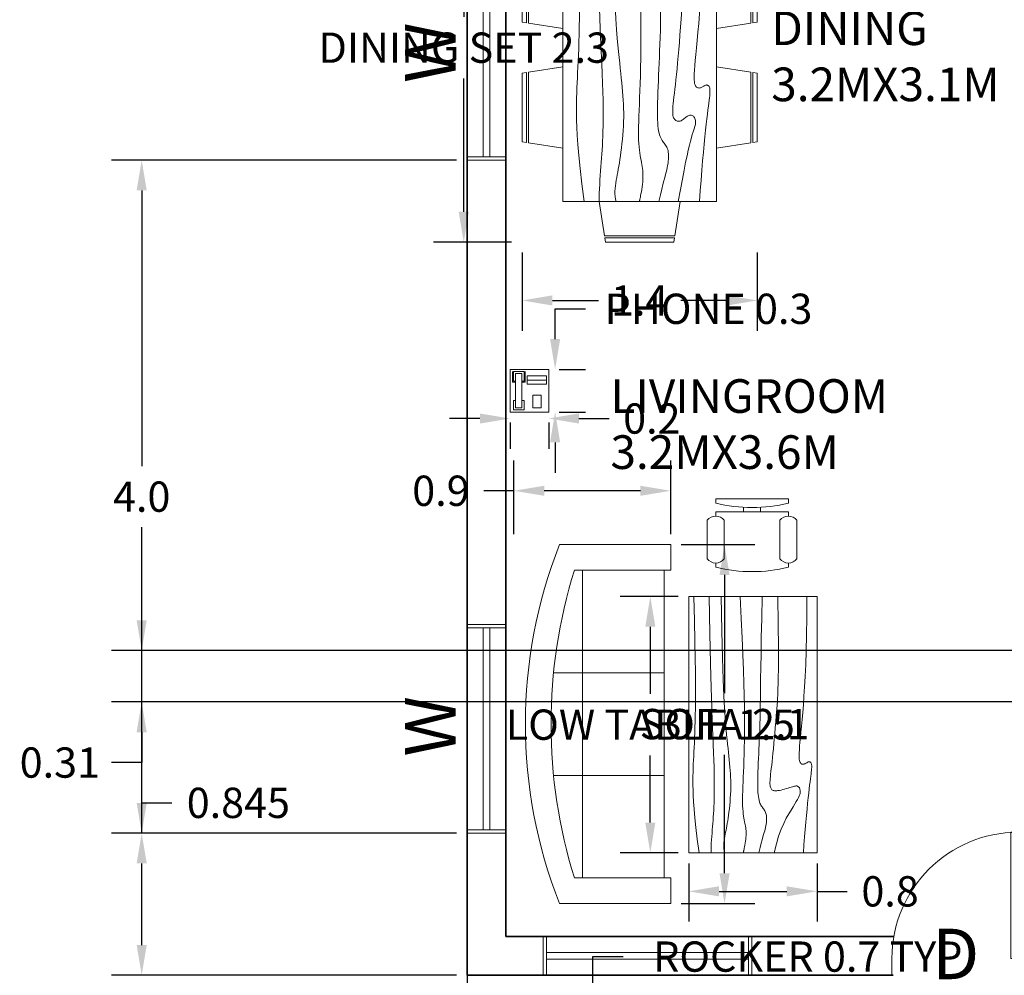
# Model space of a CAD drawing. Units: metres. Extents: x 40.9 to 56.1, y -1.4 to 24.2.
# Tile 3 of 7: x 42.6 to 48.4, y 12.9 to 18.6. Entities that reach past the tile are written whole.
import ezdxf

# ---------------------------------------------------------------- set-up
doc = ezdxf.new("R2010")
doc.units = ezdxf.units.M
doc.header["$MEASUREMENT"] = 0
for name, color, linetype, lineweight in [('A-ANNO-DIMS', 2, 'Continuous', 18), ('A-ANNO-TEXT', 7, 'Continuous', 18), ('A-AREA-IDEN', 7, 'Continuous', 18), ('A-DOOR', 3, 'Continuous', 18), ('A-EQPM', 8, 'Continuous', 18), ('A-FLOR', 7, 'Continuous', 25), ('A-FURN', 8, 'Continuous', 18), ('A-GLAZ', 4, 'Continuous', 18), ('A-WALL', 7, 'Continuous', 35)]:
    doc.layers.add(name, color=color, linetype=linetype, lineweight=lineweight)
doc.styles.get("Standard").update_dxf_attribs({"font": 'arial.ttf'})
doc.dimstyles.get("Standard").update_dxf_attribs({"dimtxt": 0.18, "dimasz": 0.18, "dimexe": 0.18, "dimexo": 0.0625, "dimgap": 0.09, "dimtad": 0, "dimtih": 1, "dimtoh": 1, "dimdec": 1, "dimzin": 0, "dimdsep": 46, "dimtxsty": 'Standard', "dimcen": 0.09, "dimadec": 0, "dimazin": 0, "dimtfac": 1, "dimtdec": 1, "dimtofl": 0, "dimtmove": 0, "dimatfit": 3, "dimfxl": 1, "dimtolj": 1, "dimtzin": 0, "dimarcsym": 0})

# ---------------------------------------------------------------- blocks, each defined once
blk = doc.blocks.new('*U3')
for p, q in [((-750, 0), (-750, -100)), ((0, 0), (0, -100))]:
    blk.add_line(p, q)
blk.add_lwpolyline([(0, 0), (0, 750), (-43.75, 750), (-43.75, 0)], close=True)
blk.add_arc((0, 0), 750, 90, 180)
blk = doc.blocks.new('Dining Set - 36 x 72 in.')
for p, q in [((-22.2343, 26.00059), (-23.4847, 17.99762)), ((-22.2304, 26), (-5.7608, 26)), ((-22, 27.5), (-22.1562, 26.50042)), ((-5.8416, 26.5), (-22.1534, 26.5)), ((-22, 27.5), (-6, 27.5)), ((-5.8437, 26.49966), (-6, 27.5)), ((-4.5152, 17.99762), (-5.7655, 25.99926)), ((5.7657, 26.00059), (4.5153, 17.99762)), ((5.7696, 26), (22.2392, 26)), ((6, 27.5), (5.8438, 26.50042)), ((22.1584, 26.5), (5.8466, 26.5)), ((6, 27.5), (22, 27.5)), ((22.1563, 26.49966), (22, 27.5)), ((23.4848, 17.99762), (22.2345, 25.99926)), ((36, 18), (-36, 18)), ((-36, 18), (-36, -18)), ((36, -18), (36, 18)), ((-44.0006, 8.23428), (-35.9976, 9.48474)), ((44.0006, 8.23428), (35.9976, 9.48474)), ((-45.5, 8), (-44.5004, 8.15617)), ((-45.5, 8), (-45.5, -8)), ((-44.5, -8.15843), (-44.5, 8.15338)), ((-44, 8.23041), (-44, -8.23915)), ((44, 8.23041), (44, -8.23915)), ((44.5, -8.15843), (44.5, 8.15338)), ((45.5, 8), (44.5005, 8.15617)), ((45.5, 8), (45.5, -8)), ((-44.4997, -8.15631), (-45.5, -8)), ((-35.9976, -9.48476), (-43.9993, -8.2345)), ((35.9976, -9.48476), (43.9993, -8.2345)), ((44.4997, -8.15631), (45.5, -8)), ((-36, -18), (36, -18)), ((-22.2343, -26.0006), (-23.4847, -17.99762)), ((-4.5152, -17.99762), (-5.7655, -25.99928)), ((5.7657, -26.0006), (4.5153, -17.99762)), ((23.4848, -17.99762), (22.2345, -25.99928)), ((-22.2304, -26), (-5.7608, -26)), ((-22, -27.5), (-22.1562, -26.50044)), ((-5.8416, -26.5), (-22.1534, -26.5)), ((-22, -27.5), (-6, -27.5)), ((-5.8437, -26.49967), (-6, -27.5)), ((5.7696, -26), (22.2392, -26)), ((6, -27.5), (5.8438, -26.50044)), ((22.1584, -26.5), (5.8466, -26.5)), ((6, -27.5), (22, -27.5)), ((22.1563, -26.49967), (22, -27.5))]:
    blk.add_line(p, q)
for points in [[(-36, 15), (-31.1772, 14.97754), (-26.8079, 14.91406), (-22.8538, 14.81543), (-19.276, 14.6875), (-16.0362, 14.53613), (-13.0957, 14.36718), (-10.4159, 14.18652), (-7.9583, 14), (-5.6904, 13.81315), (-3.6035, 13.63021), (-1.6954, 13.45508), (0.0365, 13.29166), (1.5945, 13.14388), (2.9811, 13.01562), (4.1988, 12.9108), (5.25, 12.83333), (6.1393, 12.78613), (6.8802, 12.76823), (7.4883, 12.77767), (7.9792, 12.8125), (8.3685, 12.87077), (8.6719, 12.95052), (8.9049, 13.0498), (9.0833, 13.16666), (9.2205, 13.29899), (9.3216, 13.44401), (9.3895, 13.59879), (9.4271, 13.76041), (9.4373, 13.92594), (9.4232, 14.09245), (9.3875, 14.257), (9.3333, 14.41666), (9.2638, 14.56917), (9.1836, 14.71484), (9.0975, 14.85465), (9.0104, 14.98958), (8.9272, 15.1206), (8.8529, 15.2487), (8.7922, 15.37483), (8.75, 15.5), (8.7305, 15.62467), (8.7344, 15.74739), (8.7617, 15.86621), (8.8125, 15.97916), (8.8867, 16.08431), (8.9844, 16.17968), (9.1055, 16.26334), (9.25, 16.33333), (9.4189, 16.38802), (9.6172, 16.42708), (9.8506, 16.45052), (10.125, 16.45833), (10.4463, 16.45052), (10.8203, 16.42708), (11.2529, 16.38802), (11.75, 16.33333), (12.3184, 16.26318), (12.9694, 16.17838), (13.7151, 16.07991), (14.5677, 15.96875), (15.5395, 15.84586), (16.6426, 15.71224), (17.8893, 15.56884), (19.2917, 15.41666), (20.859, 15.25667), (22.5879, 15.08984), (24.4721, 14.91715), (26.5052, 14.73958), (28.6809, 14.5581), (30.9929, 14.3737), (33.4347, 14.18733), (36, 14)], [(-36, 10), (-28.9766, 10.14274), (-23.1725, 10.20442), (-18.4241, 10.19775), (-14.5677, 10.13541), (-11.4399, 10.03011), (-8.877, 9.89453), (-6.7154, 9.74137), (-4.7917, 9.58333), (-2.9698, 9.43082), (-1.2246, 9.28515), (0.4415, 9.14534), (2.026, 9.01041), (3.5266, 8.87939), (4.9408, 8.7513), (6.266, 8.62516), (7.5, 8.5), (8.6411, 8.37549), (9.6914, 8.2539), (10.6538, 8.13818), (11.5312, 8.03125), (12.3267, 7.93603), (13.043, 7.85547), (13.6831, 7.79248), (14.25, 7.75), (14.7471, 7.7303), (15.1797, 7.73307), (15.5537, 7.75732), (15.875, 7.80208), (16.1494, 7.86637), (16.3828, 7.94922), (16.5811, 8.04964), (16.75, 8.16666), (16.8944, 8.29915), (17.0143, 8.44531), (17.1089, 8.60319), (17.1771, 8.77083), (17.218, 8.94629), (17.2305, 9.1276), (17.2137, 9.31282), (17.1667, 9.5), (17.0895, 9.6875), (16.987, 9.875), (16.8649, 10.0625), (16.7292, 10.25), (16.5856, 10.4375), (16.4401, 10.625), (16.2985, 10.8125), (16.1667, 11), (16.05, 11.18733), (15.9518, 11.3737), (15.8752, 11.5581), (15.8229, 11.73958), (15.798, 11.91715), (15.8034, 12.08984), (15.842, 12.25667), (15.9167, 12.41666), (16.0295, 12.56836), (16.1784, 12.70833), (16.3605, 12.83268), (16.5729, 12.9375), (16.8127, 13.01888), (17.0768, 13.07291), (17.3625, 13.0957), (17.6667, 13.08333), (17.9894, 13.03312), (18.3418, 12.94726), (18.7382, 12.82918), (19.1927, 12.68229), (19.7195, 12.51001), (20.3327, 12.31575), (21.0465, 12.10294), (21.875, 11.875), (22.8357, 11.63354), (23.959, 11.37304), (25.2786, 11.08618), (26.8282, 10.76562), (28.6414, 10.40405), (30.752, 9.99414), (33.1936, 9.52856), (36, 9)], [(-36, 5.5), (-30.7157, 5.3348), (-26.069, 5.20963), (-21.9946, 5.11767), (-18.4271, 5.05208), (-15.3009, 5.00602), (-12.5508, 4.97265), (-10.1112, 4.94515), (-7.9167, 4.91666), (-5.909, 4.88167), (-4.0586, 4.83984), (-2.3429, 4.79215), (-0.7396, 4.73958), (0.7739, 4.6831), (2.22, 4.6237), (3.6213, 4.56233), (5, 4.5), (6.373, 4.43782), (7.7344, 4.3776), (9.0723, 4.32129), (10.375, 4.27083), (11.6309, 4.22819), (12.8281, 4.19531), (13.9551, 4.17415), (15, 4.16666), (15.954, 4.17448), (16.819, 4.19791), (17.6001, 4.23698), (18.3021, 4.29166), (18.9299, 4.36198), (19.4883, 4.44791), (19.9823, 4.54948), (20.4167, 4.66666), (20.7969, 4.79899), (21.1302, 4.94401), (21.4245, 5.09879), (21.6875, 5.26041), (21.9271, 5.42594), (22.1511, 5.59245), (22.3672, 5.757), (22.5834, 5.91666), (22.8065, 6.06868), (23.0404, 6.21093), (23.2879, 6.34147), (23.5521, 6.45833), (23.8358, 6.55957), (24.142, 6.64323), (24.4735, 6.70735), (24.8334, 6.75), (25.2235, 6.76969), (25.642, 6.76692), (26.0858, 6.74267), (26.5521, 6.69791), (27.0379, 6.63362), (27.5404, 6.55078), (28.0565, 6.45036), (28.5834, 6.33333), (29.1242, 6.19987), (29.7071, 6.04687), (30.3661, 5.87044), (31.1354, 5.66666), (32.0493, 5.43164), (33.142, 5.16146), (34.4475, 4.85221), (36, 4.5)], [(-36, -1), (-30.7915, -0.6591), (-26.0195, -0.38216), (-21.6519, -0.16284), (-17.6563, 0.00521), (-14.0005, 0.12833), (-10.6523, 0.21289), (-7.5796, 0.26522), (-4.75, 0.29166), (-2.134, 0.29793), (0.2878, 0.28711), (2.5317, 0.26163), (4.6146, 0.22396), (6.5529, 0.17651), (8.3633, 0.12174), (10.0623, 0.06209), (11.6667, 0), (13.1899, -0.06201), (14.6341, -0.1211), (15.9982, -0.17432), (17.2813, -0.21875), (18.4823, -0.25147), (19.6003, -0.26953), (20.6343, -0.27002), (21.5834, -0.25), (22.4481, -0.20768), (23.2357, -0.14584), (23.9549, -0.06836), (24.6146, 0.02083), (25.2235, 0.11784), (25.7904, 0.21875), (26.3241, 0.31966), (26.8334, 0.41666), (27.3265, 0.50618), (27.8099, 0.58593), (28.2894, 0.65397), (28.7709, 0.70833), (29.2601, 0.74707), (29.763, 0.76823), (30.2855, 0.76985), (30.8334, 0.75), (31.4088, 0.70784), (31.9994, 0.64713), (32.589, 0.57275), (33.1615, 0.48958), (33.7008, 0.4025), (34.1908, 0.3164), (34.6153, 0.23616), (34.9584, 0.16666), (35.2099, 0.11165), (35.3848, 0.07031), (35.504, 0.04069), (35.5886, 0.02083), (35.6594, 0.00879), (35.7377, 0.0026), (35.8442, 0.00032), (36, 0)], [(-36, -6.5), (-27.1843, -6.31267), (-20.084, -6.1263), (-14.469, -5.9419), (-10.1094, -5.76042), (-6.7752, -5.58285), (-4.2363, -5.41016), (-2.2629, -5.24333), (-0.625, -5.08334), (0.8708, -4.93099), (2.2715, -4.78646), (3.5872, -4.64974), (4.8281, -4.52084), (6.0046, -4.39974), (7.127, -4.28646), (8.2053, -4.18099), (9.25, -4.08334), (10.2705, -3.99382), (11.2734, -3.91407), (12.2647, -3.84603), (13.25, -3.79167), (14.2354, -3.75293), (15.2266, -3.73177), (16.2295, -3.73015), (17.25, -3.75), (18.2912, -3.79248), (19.3451, -3.85547), (20.4009, -3.93604), (21.4479, -4.03125), (22.4754, -4.13819), (23.4727, -4.25391), (24.4289, -4.37549), (25.3334, -4.5), (26.1785, -4.62492), (26.9694, -4.74935), (27.7145, -4.87281), (28.4219, -4.99479), (29.1, -5.11483), (29.7572, -5.23242), (30.4016, -5.34709), (31.0417, -5.45834), (31.6837, -5.56437), (32.3262, -5.65821), (32.9658, -5.73153), (33.599, -5.77604), (34.2224, -5.78345), (34.8327, -5.74545), (35.4264, -5.65373), (36, -5.5)], [(-36, -10), (-26.4022, -9.81299), (-18.4675, -9.62891), (-11.9839, -9.45069), (-6.7396, -9.28125), (-2.5226, -9.12354), (0.8789, -8.98047), (3.6769, -8.85498), (6.0833, -8.75), (8.2767, -8.66765), (10.3021, -8.60677), (12.1712, -8.56543), (13.8958, -8.54167), (15.4876, -8.53353), (16.9583, -8.53907), (18.3197, -8.55632), (19.5834, -8.58334), (20.7616, -8.61841), (21.8685, -8.66081), (22.9188, -8.71004), (23.9271, -8.76563), (24.9081, -8.82707), (25.8763, -8.89388), (26.8465, -8.96558), (27.8334, -9.04167), (28.8474, -9.12118), (29.8828, -9.20117), (30.93, -9.27824), (31.9792, -9.34896), (33.0205, -9.40991), (34.0443, -9.45768), (35.0407, -9.48885), (36, -9.5)], [(-36, -14.5), (-30.0881, -14.33513), (-25.0332, -14.21224), (-20.7312, -14.12647), (-17.0781, -14.07292), (-13.97, -14.04671), (-11.3027, -14.04297), (-8.9724, -14.05681), (-6.875, -14.08334), (-4.9224, -14.11833), (-3.0905, -14.16016), (-1.3709, -14.20785), (0.2448, -14.26042), (1.7647, -14.3169), (3.1973, -14.3763), (4.5507, -14.43767), (5.8333, -14.5), (7.0554, -14.5621), (8.235, -14.62175), (9.3922, -14.67652), (10.5469, -14.72396), (11.7192, -14.76164), (12.929, -14.78711), (14.1965, -14.79794), (15.5417, -14.79167), (16.9933, -14.76424), (18.6152, -14.70508), (20.4804, -14.60197), (22.6615, -14.44271), (25.2312, -14.21509), (28.2624, -13.9069), (31.8277, -13.50594), (36, -13)]]:
    blk.add_lwpolyline(points)
blk = doc.blocks.new('Sofa - Roundback 7 ft.')
for p, q in [((-12.00002, -32.4421), (-12.00003, -6.5971)), ((11.99997, -32.4421), (11.99998, -6.5971)), ((-36.000027, -34), (-36.000027, -11.4696)), ((35.99998, -34), (35.99998, -11.4696)), ((-35.999844, -13.3819), (35.9998, -13.3819)), ((-36.000027, -32.4421), (35.99998, -32.4421))]:
    blk.add_line(p, q)
for points in [[(-36.000027, -34), (-42.000027, -34), (-42.000027, -8)], [(41.99998, -8), (41.99998, -34), (35.99998, -34)]]:
    blk.add_lwpolyline(points)
for centre, radius, start, end in [((0, -114.25), 114.25, 68.43141, 111.5686), ((-0.00001, -127.1968), 121.1968, 72.72033, 107.2797)]:
    blk.add_arc(centre, radius, start, end)
blk = doc.blocks.new('Table - Rectangular Woodgrain 60 x 30 in.')
for p, q in [((0, 0), (0, -30)), ((60, 0), (0, 0)), ((60, -30), (60, 0)), ((0, -30), (60, -30))]:
    blk.add_line(p, q)
for points in [[(0, -2.4), (4.8155, -2.418), (9.0302, -2.4688), (12.709, -2.5477), (15.9167, -2.65), (18.7181, -2.7711), (21.1781, -2.9063), (23.3616, -3.0508), (25.3333, -3.2), (27.1477, -3.3495), (28.8172, -3.4958), (30.3437, -3.636), (31.7291, -3.7667), (32.9756, -3.8849), (34.0849, -3.9875), (35.059, -4.0714), (35.9, -4.1334), (36.6114, -4.1711), (37.2041, -4.1854), (37.6906, -4.1779), (38.0833, -4.15), (38.3948, -4.1034), (38.6375, -4.0396), (38.8239, -3.9602), (38.9666, -3.8667), (39.0764, -3.7608), (39.1573, -3.6448), (39.2116, -3.521), (39.2416, -3.3917), (39.2498, -3.2593), (39.2385, -3.1261), (39.21, -2.9944), (39.1666, -2.8667), (39.111, -2.7447), (39.0468, -2.6281), (38.978, -2.5163), (38.9083, -2.4083), (38.8418, -2.3035), (38.7823, -2.201), (38.7337, -2.1001), (38.7, -2), (38.6844, -1.9003), (38.6875, -1.8021), (38.7094, -1.707), (38.75, -1.6167), (38.8094, -1.5326), (38.8875, -1.4563), (38.9844, -1.3893), (39.1, -1.3333), (39.2351, -1.2896), (39.3937, -1.2583), (39.5804, -1.2396), (39.8, -1.2333), (40.057, -1.2396), (40.3562, -1.2583), (40.7023, -1.2896), (41.1, -1.3333), (41.5547, -1.3895), (42.0755, -1.4573), (42.6721, -1.5361), (43.3542, -1.625), (44.1316, -1.7233), (45.014, -1.8302), (46.0114, -1.9449), (47.1333, -2.0667), (48.3862, -2.1947), (49.7625, -2.3281), (51.2513, -2.4663), (52.8416, -2.6083), (54.5226, -2.7535), (56.2833, -2.9011), (58.1127, -3.0501), (60, -3.2)], [(0, -9.2), (6.5759, -9.0858), (11.9385, -9.0365), (16.2527, -9.0418), (19.6833, -9.0917), (22.3952, -9.1759), (24.5531, -9.2844), (26.322, -9.4069), (27.8666, -9.5333), (29.3241, -9.6553), (30.7203, -9.7719), (32.0532, -9.8837), (33.3208, -9.9917), (34.5213, -10.0965), (35.6526, -10.199), (36.7128, -10.2999), (37.7, -10.4), (38.6129, -10.4996), (39.4531, -10.5969), (40.223, -10.6895), (40.925, -10.775), (41.5613, -10.8512), (42.1344, -10.9156), (42.6465, -10.966), (43.1, -11), (43.4976, -11.0158), (43.8437, -11.0136), (44.143, -10.9942), (44.4, -10.9583), (44.6195, -10.9069), (44.8062, -10.8406), (44.9648, -10.7603), (45.1, -10.6667), (45.2155, -10.5598), (45.3114, -10.4365), (45.3871, -10.2929), (45.4416, -10.125), (45.4743, -9.929), (45.4844, -9.7011), (45.4709, -9.4371), (45.4333, -9.1333), (45.3716, -8.7883), (45.2896, -8.4104), (45.1919, -8.0107), (45.0833, -7.6), (44.9685, -7.1893), (44.8521, -6.7896), (44.7388, -6.4117), (44.6333, -6.0667), (44.54, -5.7628), (44.4614, -5.4979), (44.4001, -5.2675), (44.3583, -5.0667), (44.3384, -4.8909), (44.3427, -4.7354), (44.3736, -4.5956), (44.4333, -4.4667), (44.5236, -4.3453), (44.6427, -4.2333), (44.7884, -4.1339), (44.9583, -4.05), (45.1501, -3.9849), (45.3614, -3.9417), (45.59, -3.9234), (45.8333, -3.9333), (46.0915, -3.9749), (46.3734, -4.0531), (46.6906, -4.1736), (47.0542, -4.3417), (47.4756, -4.5629), (47.9661, -4.8427), (48.5372, -5.1866), (49.2, -5.6), (49.9676, -6.0844), (50.8594, -6.625), (51.8965, -7.2031), (53.1, -7.8), (54.491, -8.3969), (56.0906, -8.975), (57.9199, -9.5156), (60, -10)], [(0, -12.8), (5.1847, -12.9322), (9.6213, -13.0323), (13.3963, -13.1059), (16.5958, -13.1583), (19.3063, -13.1952), (21.614, -13.2219), (23.6054, -13.2439), (25.3666, -13.2667), (26.9728, -13.2947), (28.4531, -13.3281), (29.8256, -13.3663), (31.1083, -13.4083), (32.3191, -13.4535), (33.476, -13.501), (34.597, -13.5501), (35.7, -13.6), (36.7984, -13.6497), (37.8875, -13.6979), (38.9578, -13.743), (40, -13.7833), (41.0047, -13.8174), (41.9625, -13.8438), (42.864, -13.8607), (43.7, -13.8667), (44.4631, -13.8604), (45.1552, -13.8417), (45.7801, -13.8104), (46.3416, -13.7667), (46.8439, -13.7104), (47.2906, -13.6417), (47.6858, -13.5604), (48.0333, -13.4667), (48.3375, -13.3608), (48.6042, -13.2448), (48.8396, -13.121), (49.05, -12.9917), (49.2417, -12.8593), (49.4208, -12.7261), (49.5937, -12.5944), (49.7667, -12.4667), (49.9452, -12.3451), (50.1323, -12.2313), (50.3303, -12.1268), (50.5416, -12.0333), (50.7686, -11.9524), (51.0135, -11.8854), (51.2788, -11.8341), (51.5666, -11.8), (51.8785, -11.7843), (52.2116, -11.7865), (52.562, -11.8059), (52.926, -11.8417), (53.2998, -11.8931), (53.6795, -11.9594), (54.0614, -12.0397), (54.4416, -12.1333), (54.8223, -12.2401), (55.2293, -12.3625), (55.6942, -12.5037), (56.2489, -12.6667), (56.9251, -12.8547), (57.7545, -13.0708), (58.7689, -13.3182), (60, -13.6)], [(0, -18), (5.124, -17.7273), (9.6609, -17.5057), (13.6705, -17.3303), (17.2125, -17.1958), (20.3467, -17.0973), (23.1328, -17.0297), (25.6307, -16.9878), (27.9, -16.9667), (29.9928, -16.9617), (31.9302, -16.9703), (33.7254, -16.9907), (35.3917, -17.0208), (36.9423, -17.0588), (38.3906, -17.1026), (39.7499, -17.1503), (41.0333, -17.2), (42.2519, -17.2496), (43.4073, -17.2969), (44.4986, -17.3395), (45.525, -17.375), (46.4858, -17.4012), (47.3802, -17.4156), (48.2074, -17.416), (48.9667, -17.4), (49.6583, -17.3662), (50.2872, -17.3167), (50.8595, -17.2547), (51.3812, -17.1833), (51.8584, -17.1057), (52.2971, -17.025), (52.7034, -16.9443), (53.0833, -16.8667), (53.443, -16.7951), (53.789, -16.7313), (54.128, -16.6768), (54.4666, -16.6334), (54.8115, -16.6024), (55.1693, -16.5854), (55.5465, -16.5841), (55.95, -16.6), (56.3828, -16.6337), (56.8346, -16.6823), (57.2915, -16.7418), (57.7396, -16.8084), (58.165, -16.878), (58.5539, -16.9469), (58.8924, -17.0111), (59.1666, -17.0667), (59.3679, -17.1107), (59.5078, -17.1438), (59.6032, -17.1675), (59.6708, -17.1833), (59.7275, -17.193), (59.7901, -17.1979), (59.8753, -17.1998), (60, -17.2)], [(0, -22.4), (8.0098, -22.2501), (14.4094, -22.1011), (19.4168, -21.9535), (23.25, -21.8083), (26.1269, -21.6663), (28.2656, -21.5281), (29.884, -21.3947), (31.2, -21.2667), (32.3967, -21.1448), (33.5172, -21.0292), (34.5697, -20.9198), (35.5625, -20.8167), (36.5037, -20.7198), (37.4015, -20.6292), (38.2642, -20.5448), (39.1, -20.4667), (39.9164, -20.3951), (40.7187, -20.3313), (41.5117, -20.2768), (42.3, -20.2333), (43.0883, -20.2024), (43.8812, -20.1854), (44.6836, -20.1841), (45.5, -20.2), (46.3328, -20.234), (47.1747, -20.2844), (48.0163, -20.3488), (48.8479, -20.425), (49.66, -20.5106), (50.4429, -20.6031), (51.1872, -20.7004), (51.8833, -20.8), (52.5246, -20.8999), (53.1166, -20.9995), (53.6681, -21.0983), (54.1875, -21.1958), (54.6834, -21.2919), (55.1646, -21.3859), (55.6394, -21.4777), (56.1167, -21.5667), (56.6028, -21.6515), (57.0961, -21.7266), (57.5929, -21.7852), (58.0896, -21.8208), (58.5823, -21.8268), (59.0674, -21.7964), (59.5412, -21.723), (60, -21.6)], [(0, -25.2), (8.6355, -25.0504), (15.7026, -24.9031), (21.4049, -24.7606), (25.9458, -24.625), (29.529, -24.4988), (32.3578, -24.3844), (34.6359, -24.284), (36.5667, -24.2), (38.3213, -24.1341), (39.9417, -24.0854), (41.437, -24.0523), (42.8167, -24.0333), (44.0901, -24.0268), (45.2667, -24.0313), (46.3557, -24.0451), (47.3667, -24.0667), (48.309, -24.0947), (49.1928, -24.1287), (50.0284, -24.168), (50.826, -24.2125), (51.5959, -24.2617), (52.3483, -24.3151), (53.0935, -24.3725), (53.8417, -24.4334), (54.6009, -24.497), (55.3699, -24.561), (56.1454, -24.6226), (56.9239, -24.6792), (57.7021, -24.7279), (58.4764, -24.7662), (59.2435, -24.7911), (60, -24.8)], [(0, -28.8), (5.6867, -28.6681), (10.45, -28.5698), (14.407, -28.5012), (17.675, -28.4584), (20.3711, -28.4374), (22.6125, -28.4344), (24.5164, -28.4455), (26.2, -28.4667), (27.762, -28.4947), (29.2276, -28.5281), (30.6033, -28.5663), (31.8958, -28.6084), (33.1118, -28.6535), (34.2578, -28.7011), (35.3405, -28.7501), (36.3666, -28.8), (37.3443, -28.8497), (38.288, -28.8974), (39.2137, -28.9412), (40.1375, -28.9792), (41.0753, -29.0093), (42.0432, -29.0297), (43.0572, -29.0384), (44.1333, -29.0333), (45.2936, -29.0114), (46.5843, -28.9641), (48.0579, -28.8816), (49.7666, -28.7542), (51.7629, -28.5721), (54.0989, -28.3255), (56.8272, -28.0048), (60, -27.6)]]:
    blk.add_lwpolyline(points)
blk = doc.blocks.new('Phone - Desk')
for p, q in [((-4.5, -5), (-4.5, 5)), ((-4.5, 5), (4.5, 5)), ((4.5, 5), (4.5, -5)), ((-4, 4.5), (-4, 2)), ((-3.75, 4.5), (-3.75, 2.25)), ((-1.25, 4.5), (-3.75, 4.5)), ((-3.25, 4), (-3.25, -4)), ((-3.25, 4), (-1.75, 4)), ((-1.75, -4), (-1.75, 4)), ((-1.25, 2.25), (-1.25, 4.5)), ((-1, 2), (-1, 4.5)), ((4, 3.5), (-0.5, 3.5)), ((-0.5, 3.5), (-0.5, 1.5)), ((-0.5, 2.5), (4, 2.5)), ((4, 1.5), (4, 3.5)), ((-4, 2), (-3.25, 2)), ((-3.75, 2.25), (-3.25, 2.25)), ((-1.75, 2.25), (-1.25, 2.25)), ((-1.75, 2), (-1, 2)), ((-0.5, 1.5), (4, 1.5)), ((-3.75, -2.25), (-3.25, -2.25)), ((-3.75, -4.5), (-3.75, -2.25)), ((-1.75, -2.25), (-1.25, -2.25)), ((-1.25, -2.25), (-1.25, -4.5)), ((2.75, -1), (0.75, -1)), ((0.75, -1), (0.75, -4)), ((2.75, -4), (2.75, -1)), ((-1.25, -4.5), (-3.75, -4.5)), ((-3.25, -4), (-1.75, -4)), ((0.75, -4), (2.75, -4)), ((4.5, -5), (-4.5, -5))]:
    blk.add_line(p, q)
blk = doc.blocks.new('Chair - Desk')
for p, q in [((-8.5, 0), (-8.5, -1)), ((-8.5, 0), (8.5, 0)), ((8.5, 0), (8.5, -1)), ((-2, -3), (-2, -1.9355)), ((2, -1.9576), (2, -3)), ((-8.5, -3), (-8.5, -4)), ((-8.5, -3), (8.5, -3)), ((8.5, -3), (8.5, -4)), ((-10.5, -5), (-10.5, -14)), ((-6.5, -14), (-6.5, -5)), ((6.5, -5), (6.5, -14)), ((10.5, -14), (10.5, -5)), ((-8.5, -15), (-8.5, -16)), ((8.5, -15), (8.5, -16))]:
    blk.add_line(p, q)
for centre, radius, start, end in [((0, 34.625), 36.625, 256.5803, 283.4197), ((-8.5, -6.5), 2.5, 36.8699, 143.1301), ((8.5, -6.5), 2.5, 36.8699, 143.1301), ((-8.5, -12.5), 2.5, 216.8699, 323.1301), ((0, 19.625), 36.625, 256.5803, 283.4197), ((8.5, -12.5), 2.5, 216.8699, 323.1301)]:
    blk.add_arc(centre, radius, start, end)
blk = doc.blocks.new('WIN-1200-PLAN')
for p, q in [((-0.0002, 0.0003), (-0.0002, 0.2303)), ((0.0198, 0.0003), (0.0198, 0.2303)), ((1.2198, 0.0003), (1.2198, 0.2303)), ((1.2398, 0.0003), (1.2398, 0.2303)), ((0.0198, 0.1353), (1.2198, 0.1353)), ((0.0198, 0.0953), (1.2198, 0.0953))]:
    blk.add_line(p, q)
blk = doc.blocks.new('*D87')
at = {"layer": 'A-ANNO-DIMS', "color": 0, "lineweight": -2, "transparency": 16777216}
for p, q in [((46.0031, 12.8585), (46.0031, 13.0385)), ((46.0031, 13.0385), (46.1831, 13.0385)), ((45.9627, 12.8585), (46.1831, 12.8585)), ((46.0031, 12.3527), (46.0031, 12.6785)), ((45.9627, 12.1727), (46.1831, 12.1727))]:
    blk.add_line(p, q, dxfattribs=at)
at = {"layer": 'A-ANNO-DIMS', "color": 0, "transparency": 16777216}
for points in [[(45.9731, 12.6785), (46.0331, 12.6785), (46.0031, 12.8585)], [(45.9731, 12.3527), (46.0331, 12.3527), (46.0031, 12.1727)]]:
    blk.add_solid(points, dxfattribs=at)
at = {"layer": 'Defpoints', "color": 0, "transparency": 16777216}
for p in [(45.9002, 12.8585), (46.0031, 12.8585), (45.9002, 12.1727)]:
    blk.add_point(p, dxfattribs=at)
at = {"layer": 'A-ANNO-DIMS', "color": 0, "transparency": 16777216, "insert": (47.3143, 13.0385), "char_height": 0.18, "attachment_point": 5}
blk.add_mtext('\\A1;ROCKER 0.7 TYP.', dxfattribs=at)
blk = doc.blocks.new('*D97')
at = {"layer": 'A-ANNO-DIMS', "color": 0, "lineweight": -2, "transparency": 16777216}
for p, q in [((45.52, 19.5966), (45.0558, 19.5966)), ((45.2358, 19.4166), (45.2358, 18.624)), ((45.2358, 17.4652), (45.2358, 18.2578)), ((45.52, 17.2852), (45.0558, 17.2852))]:
    blk.add_line(p, q, dxfattribs=at)
at = {"layer": 'A-ANNO-DIMS', "color": 0, "transparency": 16777216}
for points in [[(45.2058, 19.4166), (45.2658, 19.4166), (45.2358, 19.5966)], [(45.2058, 17.4652), (45.2658, 17.4652), (45.2358, 17.2852)]]:
    blk.add_solid(points, dxfattribs=at)
at = {"layer": 'Defpoints', "color": 0, "transparency": 16777216}
for p in [(45.5825, 19.5966), (45.2358, 17.2852), (45.5825, 17.2852)]:
    blk.add_point(p, dxfattribs=at)
at = {"layer": 'A-ANNO-DIMS', "color": 0, "transparency": 16777216, "insert": (45.2358, 18.4409), "char_height": 0.18, "attachment_point": 5}
blk.add_mtext('\\A1;DINING SET 2.3', dxfattribs=at)
blk = doc.blocks.new('*D98')
at = {"layer": 'A-ANNO-DIMS', "color": 0, "lineweight": -2, "transparency": 16777216}
for p, q in [((45.5825, 17.2227), (45.5825, 16.7585)), ((46.9795, 17.2227), (46.9795, 16.7585)), ((45.7625, 16.9385), (46.036, 16.9385)), ((46.7995, 16.9385), (46.526, 16.9385))]:
    blk.add_line(p, q, dxfattribs=at)
at = {"layer": 'A-ANNO-DIMS', "color": 0, "transparency": 16777216}
for points in [[(45.7625, 16.9685), (45.7625, 16.9085), (45.5825, 16.9385)], [(46.7995, 16.9685), (46.7995, 16.9085), (46.9795, 16.9385)]]:
    blk.add_solid(points, dxfattribs=at)
at = {"layer": 'Defpoints', "color": 0, "transparency": 16777216}
for p in [(45.5825, 17.2852), (46.9795, 17.2852), (46.9795, 16.9385)]:
    blk.add_point(p, dxfattribs=at)
at = {"layer": 'A-ANNO-DIMS', "color": 0, "transparency": 16777216, "insert": (46.281, 16.9385), "char_height": 0.18, "attachment_point": 5}
blk.add_mtext('\\A1;1.4', dxfattribs=at)
blk = doc.blocks.new('*D99')
at = {"layer": 'A-ANNO-DIMS', "color": 0, "lineweight": -2, "transparency": 16777216}
for p, q in [((46.5281, 15.4873), (46.9656, 15.4873)), ((46.7856, 15.3073), (46.7856, 14.6036)), ((46.7856, 13.5337), (46.7856, 14.2373)), ((46.5281, 13.3537), (46.9656, 13.3537))]:
    blk.add_line(p, q, dxfattribs=at)
at = {"layer": 'A-ANNO-DIMS', "color": 0, "transparency": 16777216}
for points in [[(46.7556, 15.3073), (46.8156, 15.3073), (46.7856, 15.4873)], [(46.7556, 13.5337), (46.8156, 13.5337), (46.7856, 13.3537)]]:
    blk.add_solid(points, dxfattribs=at)
at = {"layer": 'Defpoints', "color": 0, "transparency": 16777216}
for p in [(46.4656, 15.4873), (46.7856, 15.4873), (46.4656, 13.3537)]:
    blk.add_point(p, dxfattribs=at)
at = {"layer": 'A-ANNO-DIMS', "color": 0, "transparency": 16777216, "insert": (46.7856, 14.4205), "char_height": 0.18, "attachment_point": 5}
blk.add_mtext('\\A1;SOFA 2.1', dxfattribs=at)
blk = doc.blocks.new('*D100')
at = {"layer": 'A-ANNO-DIMS', "color": 0, "lineweight": -2, "transparency": 16777216}
for p, q in [((45.5343, 15.5498), (45.5343, 15.9873)), ((46.4656, 15.5498), (46.4656, 15.9873)), ((45.5343, 15.8073), (45.3543, 15.8073)), ((46.2856, 15.8073), (45.7143, 15.8073))]:
    blk.add_line(p, q, dxfattribs=at)
at = {"layer": 'A-ANNO-DIMS', "color": 0, "transparency": 16777216}
for points in [[(45.7143, 15.8373), (45.7143, 15.7773), (45.5343, 15.8073)], [(46.2856, 15.8373), (46.2856, 15.7773), (46.4656, 15.8073)]]:
    blk.add_solid(points, dxfattribs=at)
at = {"layer": 'Defpoints', "color": 0, "transparency": 16777216}
for p in [(45.5343, 15.8073), (45.5343, 15.4873), (46.4656, 15.4873)]:
    blk.add_point(p, dxfattribs=at)
at = {"layer": 'A-ANNO-DIMS', "color": 0, "transparency": 16777216, "insert": (45.1002, 15.8073), "char_height": 0.18, "attachment_point": 5}
blk.add_mtext('\\A1;0.9', dxfattribs=at)
blk = doc.blocks.new('*D101')
at = {"layer": 'A-ANNO-DIMS', "color": 0, "lineweight": -2, "transparency": 16777216}
for p, q in [((46.5105, 15.179), (46.1644, 15.179)), ((46.3444, 14.999), (46.3444, 14.6001)), ((46.3444, 13.835), (46.3444, 14.2338)), ((46.5105, 13.655), (46.1644, 13.655))]:
    blk.add_line(p, q, dxfattribs=at)
at = {"layer": 'A-ANNO-DIMS', "color": 0, "transparency": 16777216}
for points in [[(46.3144, 14.999), (46.3744, 14.999), (46.3444, 15.179)], [(46.3144, 13.835), (46.3744, 13.835), (46.3444, 13.655)]]:
    blk.add_solid(points, dxfattribs=at)
at = {"layer": 'Defpoints', "color": 0, "transparency": 16777216}
for p in [(46.573, 15.179), (46.3444, 13.655), (46.573, 13.655)]:
    blk.add_point(p, dxfattribs=at)
at = {"layer": 'A-ANNO-DIMS', "color": 0, "transparency": 16777216, "insert": (46.3444, 14.417), "char_height": 0.18, "attachment_point": 5}
blk.add_mtext('\\A1;LOW TABLE 1.5', dxfattribs=at)
blk = doc.blocks.new('*D102')
at = {"layer": 'A-ANNO-DIMS', "color": 0, "lineweight": -2, "transparency": 16777216}
for p, q in [((46.573, 13.5925), (46.573, 13.2464)), ((47.335, 13.5925), (47.335, 13.2464)), ((46.753, 13.4264), (47.155, 13.4264)), ((47.335, 13.4264), (47.515, 13.4264))]:
    blk.add_line(p, q, dxfattribs=at)
at = {"layer": 'A-ANNO-DIMS', "color": 0, "transparency": 16777216}
for points in [[(46.753, 13.4564), (46.753, 13.3964), (46.573, 13.4264)], [(47.155, 13.4564), (47.155, 13.3964), (47.335, 13.4264)]]:
    blk.add_solid(points, dxfattribs=at)
at = {"layer": 'Defpoints', "color": 0, "transparency": 16777216}
for p in [(46.573, 13.655), (47.335, 13.655), (47.335, 13.4264)]:
    blk.add_point(p, dxfattribs=at)
at = {"layer": 'A-ANNO-DIMS', "color": 0, "transparency": 16777216, "insert": (47.7691, 13.4264), "char_height": 0.18, "attachment_point": 5}
blk.add_mtext('\\A1;0.8', dxfattribs=at)
blk = doc.blocks.new('*D115')
at = {"layer": 'A-ANNO-DIMS', "color": 0, "lineweight": -2, "transparency": 16777216}
for p, q in [((45.7787, 16.7088), (45.7787, 16.8888)), ((45.7787, 16.8888), (45.9587, 16.8888)), ((45.8031, 16.5288), (45.9587, 16.5288)), ((45.8031, 16.2748), (45.9587, 16.2748)), ((45.7787, 16.0948), (45.7787, 15.9148))]:
    blk.add_line(p, q, dxfattribs=at)
at = {"layer": 'A-ANNO-DIMS', "color": 0, "transparency": 16777216}
for points in [[(45.7487, 16.7088), (45.8087, 16.7088), (45.7787, 16.5288)], [(45.7487, 16.0948), (45.8087, 16.0948), (45.7787, 16.2748)]]:
    blk.add_solid(points, dxfattribs=at)
at = {"layer": 'Defpoints', "color": 0, "transparency": 16777216}
for p in [(45.7406, 16.5288), (45.7787, 16.5288), (45.7406, 16.2748)]:
    blk.add_point(p, dxfattribs=at)
at = {"layer": 'A-ANNO-DIMS', "color": 0, "transparency": 16777216, "insert": (46.6901, 16.8888), "char_height": 0.18, "attachment_point": 5}
blk.add_mtext('\\A1;PHONE 0.3', dxfattribs=at)
blk = doc.blocks.new('*D116')
at = {"layer": 'A-ANNO-DIMS', "color": 0, "lineweight": -2, "transparency": 16777216}
for p, q in [((45.332, 16.2367), (45.152, 16.2367)), ((45.512, 16.2123), (45.512, 16.0567)), ((45.7406, 16.2123), (45.7406, 16.0567)), ((45.9206, 16.2367), (46.1006, 16.2367))]:
    blk.add_line(p, q, dxfattribs=at)
at = {"layer": 'A-ANNO-DIMS', "color": 0, "transparency": 16777216}
for points in [[(45.332, 16.2667), (45.332, 16.2067), (45.512, 16.2367)], [(45.9206, 16.2667), (45.9206, 16.2067), (45.7406, 16.2367)]]:
    blk.add_solid(points, dxfattribs=at)
at = {"layer": 'Defpoints', "color": 0, "transparency": 16777216}
for p in [(45.512, 16.2748), (45.7406, 16.2748), (45.7406, 16.2367)]:
    blk.add_point(p, dxfattribs=at)
at = {"layer": 'A-ANNO-DIMS', "color": 0, "transparency": 16777216, "insert": (46.3535, 16.2367), "char_height": 0.18, "attachment_point": 5}
blk.add_mtext('\\A1;0.2', dxfattribs=at)
blk = doc.blocks.new('*D136')
at = {"layer": 'A-ANNO-DIMS', "color": 0, "lineweight": -2, "transparency": 16777216}
for p, q in [((48.7602, 14.8764), (48.7602, 24.2418)), ((49.4546, 14.8764), (49.4546, 24.2418)), ((48.5802, 24.0618), (48.4002, 24.0618)), ((49.6346, 24.0618), (49.8146, 24.0618))]:
    blk.add_line(p, q, dxfattribs=at)
at = {"layer": 'A-ANNO-DIMS', "color": 0, "transparency": 16777216}
for points in [[(48.5802, 24.0918), (48.5802, 24.0318), (48.7602, 24.0618)], [(49.6346, 24.0918), (49.6346, 24.0318), (49.4546, 24.0618)]]:
    blk.add_solid(points, dxfattribs=at)
at = {"layer": 'Defpoints', "color": 0, "transparency": 16777216}
for p in [(49.4546, 24.0618), (48.7602, 14.8139), (49.4546, 14.8139)]:
    blk.add_point(p, dxfattribs=at)
at = {"layer": 'A-ANNO-DIMS', "color": 0, "transparency": 16777216, "insert": (49.1074, 24.0618), "char_height": 0.18, "attachment_point": 5}
blk.add_mtext('\\A1;0.69', dxfattribs=at)
blk = doc.blocks.new('*D137')
at = {"layer": 'A-ANNO-DIMS', "color": 0, "lineweight": -2, "transparency": 16777216}
for p, q in [((43.3221, 13.7723), (43.3221, 13.9523)), ((43.3221, 13.9523), (43.5021, 13.9523)), ((45.1927, 13.7723), (43.1421, 13.7723)), ((43.3221, 13.1073), (43.3221, 13.5923)), ((45.1927, 12.9273), (43.1421, 12.9273))]:
    blk.add_line(p, q, dxfattribs=at)
at = {"layer": 'A-ANNO-DIMS', "color": 0, "transparency": 16777216}
for points in [[(43.2921, 13.5923), (43.3521, 13.5923), (43.3221, 13.7723)], [(43.2921, 13.1073), (43.3521, 13.1073), (43.3221, 12.9273)]]:
    blk.add_solid(points, dxfattribs=at)
at = {"layer": 'Defpoints', "color": 0, "transparency": 16777216}
for p in [(43.3221, 13.7723), (45.2552, 13.7723), (45.2552, 12.9273)]:
    blk.add_point(p, dxfattribs=at)
at = {"layer": 'A-ANNO-DIMS', "color": 0, "transparency": 16777216, "insert": (43.8965, 13.9523), "char_height": 0.18, "attachment_point": 5}
blk.add_mtext('\\A1;0.845', dxfattribs=at)
blk = doc.blocks.new('*D138')
at = {"layer": 'A-ANNO-DIMS', "color": 0, "lineweight": -2, "transparency": 16777216}
for p, q in [((45.1927, 17.7723), (43.1421, 17.7723)), ((43.3221, 17.5923), (43.3221, 15.9542)), ((43.3221, 13.9523), (43.3221, 15.5903)), ((45.1927, 13.7723), (43.1421, 13.7723))]:
    blk.add_line(p, q, dxfattribs=at)
at = {"layer": 'A-ANNO-DIMS', "color": 0, "transparency": 16777216}
for points in [[(43.2921, 17.5923), (43.3521, 17.5923), (43.3221, 17.7723)], [(43.2921, 13.9523), (43.3521, 13.9523), (43.3221, 13.7723)]]:
    blk.add_solid(points, dxfattribs=at)
at = {"layer": 'Defpoints', "color": 0, "transparency": 16777216}
for p in [(43.3221, 17.7723), (45.2552, 17.7723), (45.2552, 13.7723)]:
    blk.add_point(p, dxfattribs=at)
at = {"layer": 'A-ANNO-DIMS', "color": 0, "transparency": 16777216, "insert": (43.3221, 15.7723), "char_height": 0.18, "attachment_point": 5}
blk.add_mtext('\\A1;4.0', dxfattribs=at)
blk = doc.blocks.new('*D151')
at = {"layer": 'A-ANNO-DIMS', "color": 0, "lineweight": -2, "transparency": 16777216}
for p, q in [((43.3221, 15.0373), (43.3221, 15.2173)), ((49.9715, 14.8573), (43.1421, 14.8573)), ((50.5637, 14.5518), (43.1421, 14.5518)), ((43.3221, 14.3718), (43.3221, 14.1918)), ((43.3221, 14.1918), (43.1421, 14.1918))]:
    blk.add_line(p, q, dxfattribs=at)
at = {"layer": 'A-ANNO-DIMS', "color": 0, "transparency": 16777216}
for points in [[(43.2921, 15.0373), (43.3521, 15.0373), (43.3221, 14.8573)], [(43.2921, 14.3718), (43.3521, 14.3718), (43.3221, 14.5518)]]:
    blk.add_solid(points, dxfattribs=at)
at = {"layer": 'Defpoints', "color": 0, "transparency": 16777216}
for p in [(50.034, 14.8573), (43.3221, 14.5518), (50.6262, 14.5518)]:
    blk.add_point(p, dxfattribs=at)
at = {"layer": 'A-ANNO-DIMS', "color": 0, "transparency": 16777216, "insert": (42.8357, 14.1918), "char_height": 0.18, "attachment_point": 5}
blk.add_mtext('\\A1;0.31', dxfattribs=at)

msp = doc.modelspace()

# ---------------------------------------------------------------- linework, layer by layer
at = {"layer": 'A-FLOR'}
msp.add_line((45.2552, 12.9273), (45.2552, 9.9273), dxfattribs=at)
at = {"layer": 'A-WALL'}
for p, q in [((45.2552, 19.8573), (45.2552, 12.9273)), ((45.4852, 19.7073), (45.4852, 13.1573)), ((45.4852, 13.1573), (47.7916, 13.1573)), ((45.2552, 12.9273), (47.7869, 12.9273))]:
    msp.add_line(p, q, dxfattribs=at)

# ---------------------------------------------------------------- block references
at = {"layer": 'A-DOOR', "xscale": 0.001, "yscale": 0.001, "zscale": 0.001}
msp.add_blockref('*U3', (48.5302, 13.0273), dxfattribs=at)
at = {"layer": 'A-EQPM', "xscale": 0.0254, "yscale": 0.0254, "zscale": 0.0254}
msp.add_blockref('Phone - Desk', (45.6263, 16.4018), dxfattribs=at)
at = {"layer": 'A-FURN', "xscale": 0.0254, "yscale": 0.0254, "zscale": 0.0254}
for name, p, rotation in [('Dining Set - 36 x 72 in.', (46.281, 18.4409), 270), ('Sofa - Roundback 7 ft.', (45.602, 14.4205), 90), ('Table - Rectangular Woodgrain 60 x 30 in.', (47.335, 15.179), 270)]:
    msp.add_blockref(name, p, dxfattribs=dict(at, rotation=rotation))
msp.add_blockref('Chair - Desk', (46.9493, 15.7586), dxfattribs=at)
at = {"layer": 'A-GLAZ', "rotation": 89.99999999999937}
for p in [(45.4855, 17.7724), (45.4855, 13.7724)]:
    msp.add_blockref('WIN-1200-PLAN', p, dxfattribs=at)
at = {"layer": 'A-GLAZ'}
msp.add_blockref('WIN-1200-PLAN', (45.7077, 12.927), dxfattribs=at)

# ---------------------------------------------------------------- texts
at = {"layer": 'A-ANNO-TEXT'}
for p in [(45.1874, 18.2311), (45.1874, 14.2273)]:
    msp.add_text('W', height=0.3, rotation=90, dxfattribs=at).set_placement(p)
msp.add_text('D ', height=0.3, dxfattribs=at).set_placement((48.0178, 12.9043))
at = {"layer": 'A-AREA-IDEN', "char_height": 0.2, "attachment_point": 1}
for s, insert in [('DINING\\P3.2MX3.1M', (47.0631, 18.6563)), ('LIVINGROOM\\P3.2MX3.6M', (46.1076, 16.4704))]:
    msp.add_mtext_dynamic_manual_height_columns(s, width=2.030673, gutter_width=1, heights=[0], dxfattribs=dict(at, insert=insert))

# ---------------------------------------------------------------- dimensions: what is measured, and where the dimension line sits
at = {"layer": 'A-ANNO-DIMS'}
for base, p1, p2, override, picture, middle in [((49.4546, 24.0618), (48.7602, 14.8139), (49.4546, 14.8139), {"dimdec": 2, "dimlfac": 1, "dimrnd": 0, "dimzin": 0, "dimdsep": 46, "dimlunit": 2}, '*D136', (49.1074, 24.0618)), ((46.9795, 16.9385), (45.5825, 17.2852), (46.9795, 17.2852), {"dimdec": 1, "dimlfac": 1, "dimrnd": 0, "dimzin": 0, "dimdsep": 46, "dimlunit": 2}, '*D98', (46.281, 16.9385)), ((45.7406, 16.2367), (45.512, 16.2748), (45.7406, 16.2748), {"dimdec": 1, "dimlfac": 1, "dimrnd": 0, "dimzin": 0, "dimdsep": 46, "dimlunit": 2}, '*D116', (46.3535, 16.2367)), ((47.335, 13.4264), (46.573, 13.655), (47.335, 13.655), {"dimdec": 1, "dimlfac": 1, "dimrnd": 0, "dimzin": 0, "dimdsep": 46, "dimlunit": 2}, '*D102', (47.7691, 13.4264))]:
    dim = msp.add_linear_dim(base=base, p1=p1, p2=p2, dimstyle='Standard', override=override, dxfattribs=at)
    dim.commit()
    dim.dimension.update_dxf_attribs({"geometry": picture, "text_midpoint": middle})
for base, p1, p2, angle, text, picture, middle in [((45.2358, 17.2852), (45.5825, 19.5966), (45.5825, 17.2852), 270, 'DINING SET <>', '*D97', (45.2358, 18.4409)), ((45.7787, 16.5288), (45.7406, 16.2748), (45.7406, 16.5288), 90, 'PHONE <>', '*D115', (46.6901, 16.8888)), ((46.7856, 15.4873), (46.4656, 13.3537), (46.4656, 15.4873), 90, 'SOFA <>', '*D99', (46.7856, 14.4205)), ((46.3444, 13.655), (46.573, 15.179), (46.573, 13.655), 270, 'LOW TABLE <>', '*D101', (46.3444, 14.417)), ((46.0031, 12.8585), (45.9002, 12.1727), (45.9002, 12.8585), 90, 'ROCKER <> TYP.', '*D87', (47.3143, 13.0385))]:
    dim = msp.add_linear_dim(base=base, p1=p1, p2=p2, angle=angle, text=text, dimstyle='Standard', override={"dimdec": 1, "dimlfac": 1, "dimrnd": 0, "dimzin": 0, "dimdsep": 46, "dimlunit": 2}, dxfattribs=at)
    dim.commit()
    dim.dimension.update_dxf_attribs({"geometry": picture, "text_midpoint": middle})
for base, p1, p2, angle, override, picture, middle in [((43.3221, 17.7723), (45.2552, 13.7723), (45.2552, 17.7723), 90, {"dimdec": 1, "dimlfac": 1, "dimrnd": 0, "dimzin": 0, "dimdsep": 46, "dimlunit": 2}, '*D138', (43.3221, 15.7723)), ((45.5343, 15.8073), (46.4656, 15.4873), (45.5343, 15.4873), 180, {"dimdec": 1, "dimlfac": 1, "dimrnd": 0, "dimzin": 0, "dimdsep": 46, "dimlunit": 2}, '*D100', (45.1002, 15.8073)), ((43.3221, 14.5518), (50.034, 14.8573), (50.6262, 14.5518), 90, {"dimdec": 2, "dimlfac": 1, "dimrnd": 0, "dimzin": 0, "dimdsep": 46, "dimlunit": 2}, '*D151', (42.8357, 14.1918)), ((43.3221, 13.7723), (45.2552, 12.9273), (45.2552, 13.7723), 90, {"dimdec": 3, "dimlfac": 1, "dimrnd": 0, "dimzin": 0, "dimdsep": 46, "dimlunit": 2}, '*D137', (43.8965, 13.9523))]:
    dim = msp.add_linear_dim(base=base, p1=p1, p2=p2, angle=angle, dimstyle='Standard', override=override, dxfattribs=at)
    dim.commit()
    dim.dimension.update_dxf_attribs({"geometry": picture, "text_midpoint": middle})

doc.saveas('drawing.dxf')
